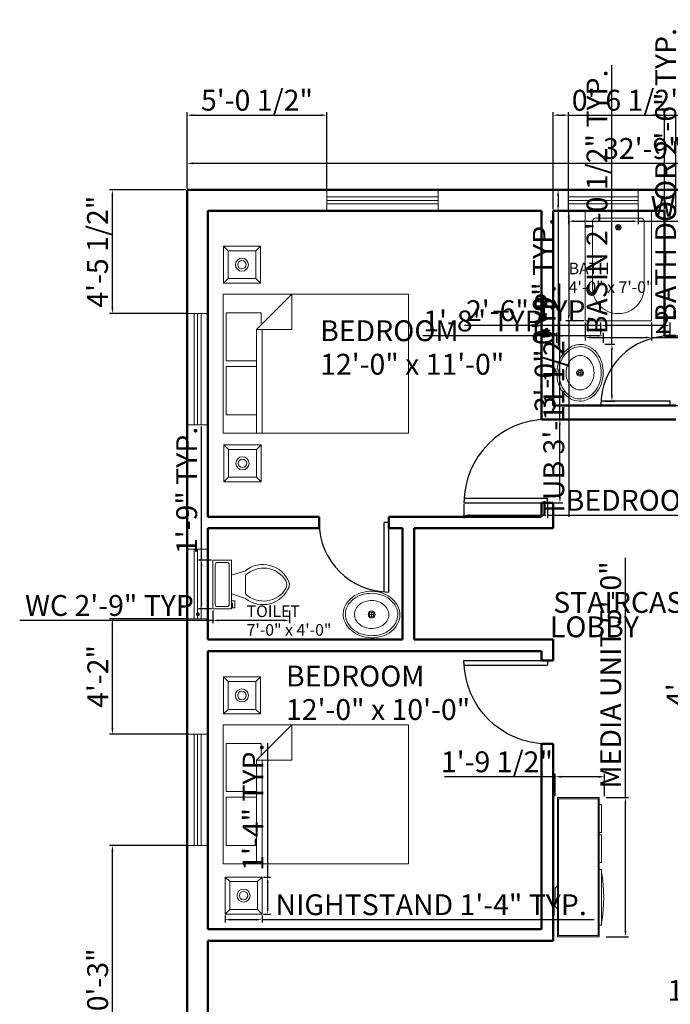
# Model space of a CAD drawing. Units: inches. Extents: x 2866 to 3545, y 873 to 1597.
# Tile 3 of 5: x 2958 to 3239, y 1172 to 1597. Entities that reach past the tile are written whole.
import ezdxf

# ---------------------------------------------------------------- set-up
doc = ezdxf.new("R2010")
doc.units = ezdxf.units.IN
doc.layers.add('A-ANNO-DIMS', color=152, linetype='Continuous', lineweight=18, true_color=0x2776bb)
for name, color, linetype, lineweight in [('A-AREA-IDEN', 7, 'Continuous', 25), ('A-DOOR', 3, 'Continuous', 25), ('A-FLOR-FIXT', 9, 'Continuous', 18), ('A-FURN', 8, 'Continuous', 18), ('A-GLAZ', 4, 'Continuous', 18), ('A-WALL', 7, 'Continuous', 50)]:
    doc.layers.add(name, color=color, linetype=linetype, lineweight=lineweight)
doc.styles.get("Standard").update_dxf_attribs({"font": 'arial.ttf'})
doc.dimstyles.new('ISO-25', dxfattribs={"dimtxt": 9, "dimasz": 2.5, "dimexe": 1.25, "dimexo": 0.625, "dimtad": 1, "dimdec": 0, "dimlunit": 3, "dimtxsty": 'Standard', "dimcen": 4.5, "dimadec": 0, "dimazin": 0, "dimtfac": 1, "dimtdec": 0, "dimtmove": 0, "dimatfit": 3, "dimfxl": 1, "dimarcsym": 0})

# ---------------------------------------------------------------- blocks, each defined once
blk = doc.blocks.new('Toilet - top')
for p, q in [((9.5, -6), (9.5, -2)), ((-8, -8.5), (-8, -8)), ((-7, -8), (-7, -9.5)), ((-4, -8), (-6, -14)), ((4, -8), (6, -14)), ((-10, -8.5), (-8, -8.5)), ((-10, -9.5), (-10, -8.5)), ((-7, -9.5), (-10, -9.5)), ((4, -14), (-4, -14))]:
    blk.add_line(p, q)
blk.add_lwpolyline([(10.5, -8), (10.5, 0), (-10.5, 0), (-10.5, -8)], close=True)
for points in [[(-9.5, -2), (-9.5, -6)], [(8.5, -1), (-8.5, -1)], [(-8.5, -7), (8.5, -7)]]:
    blk.add_lwpolyline(points)
for centre, radius, start, end in [((-8.62, -1.88), 0.884, 81.8699, 188.1301), ((8.62, -1.88), 0.884, 351.8699, 98.1301), ((-8.62, -6.12), 0.884, 171.8699, 278.1301), ((8.62, -6.12), 0.884, 261.8699, 8.1301), ((3.52, -21.58), 12.17, 141.4691, 247.9714), ((4.2, -21.82), 11.33, 136.3677, 238.9468), ((-3.52, -21.58), 12.17, 292.0284, 38.5307), ((-4.2, -21.82), 11.33, 301.053, 43.6321), ((0, -27.88), 4, 245.7318, 294.2682), ((0, -29), 4, 254.8605, 285.1395)]:
    blk.add_arc(centre, radius, start, end)
blk = doc.blocks.new('Entertainment Center')
for p, q in [((-4, 0), (-5, -1)), ((4, 0), (-4, 0)), ((5, -1), (4, 0)), ((-17, -19), (-17, -1)), ((-17, -1), (43, -1)), ((-16.5, -18.5), (-16.5, -1.5)), ((-16.5, -1.5), (42.5, -1.5)), ((42.5, -1.5), (42.5, -18.5)), ((43, -1), (43, -19)), ((43, -19), (-17, -19)), ((42.5, -18.5), (-16.5, -18.5)), ((-12, -20), (-12, -19)), ((12, -20), (-12, -20)), ((12, -19), (12, -20)), ((15, -20), (15, -19)), ((27, -20), (15, -20)), ((27, -19), (27, -20)), ((28, -20), (28, -19)), ((40, -20), (28, -20)), ((40, -19), (40, -20))]:
    blk.add_line(p, q)
blk.add_arc((0, 40), 61, 259.6111, 280.3889)
blk = doc.blocks.new('Bed - Queen')
for p, q in [((0, -80.00003), (0, 0)), ((0, 0), (59.99999, 0)), ((59.99999, 0), (59.99999, -80.00003)), ((7.99999, -1.2), (28.79998, -1.2)), ((7.99999, -14.4), (7.99999, -1.2)), ((28.79998, -1.2), (28.79998, -14.4)), ((31.19999, -1.2), (51.99999, -1.2)), ((31.19999, -14.4), (31.19999, -1.2)), ((51.99999, -1.2), (51.99999, -16.4)), ((0, -14.4), (44.8, -14.4)), ((44.8, -16.8), (0, -16.8)), ((59.99999, -29.6), (44.8, -14.4)), ((44.8, -14.4), (44.8, -29.6)), ((51.99999, -16.4), (46.79936, -16.4)), ((44.8, -29.6), (59.99999, -29.6)), ((59.99999, -80.00003), (0, -80.00003))]:
    blk.add_line(p, q)
blk = doc.blocks.new('Sink - Oval top')
for p, q in [((-1, 0), (1, 0)), ((0, 1), (0, -1))]:
    blk.add_line(p, q)
for points in [[(-12.23, 0.39, 0.117634), (-11.46, -3.36, 0.104469), (-8.88, -6.8, 0.090016), (-5.08, -9.07, 0.08192), (-0.32, -10.02, 0.08192), (4.49, -9.38, 0.090016), (8.42, -7.36, 0.104469), (11.22, -4.09, 0.117634), (12.23, -0.39, 0.117634), (11.46, 3.36, 0.104469), (8.88, 6.8, 0.090016), (5.08, 9.07, 0.08192), (0.32, 10.02, 0.08192), (-4.49, 9.38, 0.090016), (-8.42, 7.36, 0.104469), (-11.22, 4.09, 0.117634)], [(-11.29, 0.16, 0.118622), (-10.52, -3.25, 0.104678), (-8.07, -6.36, 0.089562), (-4.54, -8.37, 0.081185), (-0.13, -9.15, 0.081185), (4.3, -8.49, 0.089562), (7.89, -6.58, 0.104678), (10.42, -3.55, 0.118622), (11.29, -0.16, 0.118622), (10.52, 3.25, 0.104678), (8.07, 6.36, 0.089562), (4.54, 8.37, 0.081185), (0.13, 9.15, 0.081185), (-4.3, 8.49, 0.089562), (-7.89, 6.58, 0.104678), (-10.42, 3.55, 0.118622)], [(-7.42, 0.08, 0.118283), (-6.91, -2.17, 0.104607), (-5.29, -4.21, 0.089718), (-2.97, -5.53, 0.081436), (-0.07, -6.04, 0.081436), (2.84, -5.59, 0.089718), (5.2, -4.33, 0.104607), (6.86, -2.32, 0.118283), (7.42, -0.08, 0.118283), (6.91, 2.17, 0.104607), (5.29, 4.21, 0.089718), (2.97, 5.53, 0.081436), (0.07, 6.04, 0.081436), (-2.84, 5.59, 0.089718), (-5.2, 4.33, 0.104607), (-6.86, 2.32, 0.118283)]]:
    blk.add_lwpolyline(points, format="xyb", close=True)
for radius in [1.5, 1]:
    blk.add_circle((0, 0), radius)
blk = doc.blocks.new('Bath Tub - 26 x 60 in.')
for p, q in [((8, -18), (10, -18)), ((9, -17), (9, -19))]:
    blk.add_line(p, q)
blk.add_lwpolyline([(0, -36), (0, 0), (60, 0), (60, -36)], close=True)
for points in [[(6, -4), (42, -4)], [(4, -30), (4, -6)], [(42, -32), (6, -32)]]:
    blk.add_lwpolyline(points)
for radius in [1.5, 1]:
    blk.add_circle((9, -18), radius)
for centre, radius, start, end in [((5.75, -5.75), 1.77, 81.8699, 188.1301), ((42, -18), 14, 270, 90), ((5.75, -30.25), 1.77, 171.8699, 278.1301)]:
    blk.add_arc(centre, radius, start, end)
blk = doc.blocks.new('*D18')
at = {"layer": 'A-ANNO-DIMS', "color": 0, "lineweight": -2, "transparency": 16777216}
for p, q in [((3265.42, 1329.69), (3246.53, 1329.69)), ((3247.78, 1284.19), (3247.78, 1327.19)), ((3265.42, 1281.69), (3246.53, 1281.69))]:
    blk.add_line(p, q, dxfattribs=at)
at = {"layer": 'A-ANNO-DIMS', "color": 0, "transparency": 16777216}
for points in [[(3247.37, 1327.19), (3248.2, 1327.19), (3247.78, 1329.69)], [(3247.37, 1284.19), (3248.2, 1284.19), (3247.78, 1281.69)]]:
    blk.add_solid(points, dxfattribs=at)
at = {"layer": 'Defpoints', "color": 0, "transparency": 16777216}
for p in [(3247.78, 1329.69), (3266.04, 1329.69), (3266.04, 1281.69)]:
    blk.add_point(p, dxfattribs=at)
at = {"layer": 'A-ANNO-DIMS', "color": 0, "transparency": 16777216, "insert": (3242.66, 1305.69), "char_height": 9, "attachment_point": 5, "rotation": 90}
blk.add_mtext("4'", dxfattribs=at)
blk = doc.blocks.new('*D20')
at = {"layer": 'A-ANNO-DIMS', "color": 0, "lineweight": -2, "transparency": 16777216}
for p, q in [((3030.04, 1524.32), (3030.04, 1536.42)), ((3032.54, 1535.17), (3420.54, 1535.17)), ((3423.04, 1524.32), (3423.04, 1536.42))]:
    blk.add_line(p, q, dxfattribs=at)
at = {"layer": 'A-ANNO-DIMS', "color": 0, "transparency": 16777216}
for points in [[(3032.54, 1535.59), (3032.54, 1534.76), (3030.04, 1535.17)], [(3420.54, 1535.59), (3420.54, 1534.76), (3423.04, 1535.17)]]:
    blk.add_solid(points, dxfattribs=at)
at = {"layer": 'Defpoints', "color": 0, "transparency": 16777216}
for p in [(3423.04, 1535.17), (3030.04, 1523.69), (3423.04, 1523.69)]:
    blk.add_point(p, dxfattribs=at)
at = {"layer": 'A-ANNO-DIMS', "color": 0, "transparency": 16777216, "insert": (3226.54, 1540.4), "char_height": 9, "attachment_point": 5}
blk.add_mtext('32\'-9"', dxfattribs=at)
blk = doc.blocks.new('WIN-48IN')
for p, q in [((0, 0), (0, 48)), ((0, 48), (9, 48)), ((3, 0), (3, 48)), ((4.5, 0), (4.5, 48)), ((6, 0), (6, 48)), ((9, 48), (9, 0)), ((9, 0), (0, 0))]:
    blk.add_line(p, q)
blk = doc.blocks.new('WIN-30IN')
for p, q in [((0, 0), (0, 30)), ((0, 30), (9, 30)), ((3, 0), (3, 30)), ((4.5, 0), (4.5, 30)), ((6, 0), (6, 30)), ((9, 30), (9, 0)), ((9, 0), (0, 0))]:
    blk.add_line(p, q)
blk = doc.blocks.new('BEDSIDE-STAND-16IN')
for p, q in [((0, 16), (2, 14)), ((14, 14), (16, 16)), ((0, 0), (2, 2)), ((16, 0), (14, 2))]:
    blk.add_line(p, q)
for points in [[(0, 16), (16, 16), (16, 0), (0, 0)], [(2, 14), (14, 14), (14, 2), (2, 2)]]:
    blk.add_lwpolyline(points, close=True)
for radius in [2.82, 1.82]:
    blk.add_circle((8, 8), radius)
blk = doc.blocks.new('DOOR-SWING-30IN')
for p, q in [((0, 30), (0, 0)), ((2, 30), (2, 0)), ((0, 0), (2, 0))]:
    blk.add_line(p, q)
blk.add_arc((0, 0), 30, 0, 90)
blk = doc.blocks.new('DOOR-SWING-36IN')
for p, q in [((0, 2), (36, 2)), ((36, 0), (36, 2)), ((0, 0), (36, 0))]:
    blk.add_line(p, q)
blk.add_arc((36, 0), 36, 90, 180)
blk = doc.blocks.new('*D29')
at = {"layer": 'A-ANNO-DIMS', "color": 0, "lineweight": -2, "transparency": 16777216}
for p, q in [((3194.66, 1514.07), (3194.66, 1508.94)), ((3224.66, 1514.07), (3224.66, 1508.94)), ((3197.16, 1510.19), (3222.16, 1510.19)), ((3224.66, 1510.19), (3342.29, 1510.19))]:
    blk.add_line(p, q, dxfattribs=at)
at = {"layer": 'A-ANNO-DIMS', "color": 0, "transparency": 16777216}
for points in [[(3197.16, 1510.61), (3197.16, 1509.78), (3194.66, 1510.19)], [(3222.16, 1510.61), (3222.16, 1509.78), (3224.66, 1510.19)]]:
    blk.add_solid(points, dxfattribs=at)
at = {"layer": 'Defpoints', "color": 0, "transparency": 16777216}
for p in [(3194.66, 1514.69), (3224.66, 1514.69), (3224.66, 1510.19)]:
    blk.add_point(p, dxfattribs=at)
at = {"layer": 'A-ANNO-DIMS', "color": 0, "transparency": 16777216, "insert": (3284.73, 1515.47), "char_height": 9, "attachment_point": 5}
blk.add_mtext('WINDOW 2\'-6" TYP.', dxfattribs=at)
blk = doc.blocks.new('*D30')
at = {"layer": 'A-ANNO-DIMS', "color": 0, "lineweight": -2, "transparency": 16777216}
for p, q in [((3194.03, 1523.69), (3188.91, 1523.69)), ((3190.16, 1521.19), (3190.16, 1517.19)), ((3194.03, 1514.69), (3188.91, 1514.69)), ((3190.16, 1514.69), (3190.16, 1456.08))]:
    blk.add_line(p, q, dxfattribs=at)
at = {"layer": 'A-ANNO-DIMS', "color": 0, "transparency": 16777216}
for points in [[(3189.74, 1521.19), (3190.57, 1521.19), (3190.16, 1523.69)], [(3189.74, 1517.19), (3190.57, 1517.19), (3190.16, 1514.69)]]:
    blk.add_solid(points, dxfattribs=at)
at = {"layer": 'Defpoints', "color": 0, "transparency": 16777216}
for p in [(3194.66, 1523.69), (3190.16, 1514.69), (3194.66, 1514.69)]:
    blk.add_point(p, dxfattribs=at)
at = {"layer": 'A-ANNO-DIMS', "color": 0, "transparency": 16777216, "insert": (3184.94, 1484.14), "char_height": 9, "attachment_point": 5, "rotation": 90}
blk.add_mtext('0\'-9" TYP.', dxfattribs=at)
blk = doc.blocks.new('*D31')
at = {"layer": 'A-ANNO-DIMS', "color": 0, "lineweight": -2, "transparency": 16777216}
for p, q in [((3046.41, 1210.59), (3046.41, 1207.57)), ((3048.91, 1208.82), (3059.91, 1208.82)), ((3062.41, 1210.59), (3062.41, 1207.57)), ((3062.41, 1208.82), (3205.8, 1208.82))]:
    blk.add_line(p, q, dxfattribs=at)
at = {"layer": 'A-ANNO-DIMS', "color": 0, "transparency": 16777216}
for points in [[(3048.91, 1209.23), (3048.91, 1208.4), (3046.41, 1208.82)], [(3059.91, 1209.23), (3059.91, 1208.4), (3062.41, 1208.82)]]:
    blk.add_solid(points, dxfattribs=at)
at = {"layer": 'Defpoints', "color": 0, "transparency": 16777216}
for p in [(3046.41, 1211.22), (3062.41, 1211.22), (3062.41, 1208.82)]:
    blk.add_point(p, dxfattribs=at)
at = {"layer": 'A-ANNO-DIMS', "color": 0, "transparency": 16777216, "insert": (3135.36, 1214.1), "char_height": 9, "attachment_point": 5}
blk.add_mtext('NIGHTSTAND 1\'-4" TYP.', dxfattribs=at)
blk = doc.blocks.new('*D32')
at = {"layer": 'A-ANNO-DIMS', "color": 0, "lineweight": -2, "transparency": 16777216}
for p, q in [((3064.81, 1227.22), (3064.81, 1284.98)), ((3063.04, 1227.22), (3066.06, 1227.22)), ((3064.81, 1213.72), (3064.81, 1224.72)), ((3063.04, 1211.22), (3066.06, 1211.22))]:
    blk.add_line(p, q, dxfattribs=at)
at = {"layer": 'A-ANNO-DIMS', "color": 0, "transparency": 16777216}
for points in [[(3064.39, 1224.72), (3065.23, 1224.72), (3064.81, 1227.22)], [(3064.39, 1213.72), (3065.23, 1213.72), (3064.81, 1211.22)]]:
    blk.add_solid(points, dxfattribs=at)
at = {"layer": 'Defpoints', "color": 0, "transparency": 16777216}
for p in [(3062.41, 1227.22), (3064.81, 1227.22), (3062.41, 1211.22)]:
    blk.add_point(p, dxfattribs=at)
at = {"layer": 'A-ANNO-DIMS', "color": 0, "transparency": 16777216, "insert": (3059.66, 1257.35), "char_height": 9, "attachment_point": 5, "rotation": 90}
blk.add_mtext('1\'-4" TYP.', dxfattribs=at)
blk = doc.blocks.new('*D35')
at = {"layer": 'A-ANNO-DIMS', "color": 0, "lineweight": -2, "transparency": 16777216}
for p, q in [((3243.04, 1460.69), (3243.04, 1597.14)), ((3239.17, 1460.69), (3244.29, 1460.69)), ((3243.04, 1433.19), (3243.04, 1458.19)), ((3239.17, 1430.69), (3244.29, 1430.69))]:
    blk.add_line(p, q, dxfattribs=at)
at = {"layer": 'A-ANNO-DIMS', "color": 0, "transparency": 16777216}
for points in [[(3242.63, 1458.19), (3243.46, 1458.19), (3243.04, 1460.69)], [(3242.63, 1433.19), (3243.46, 1433.19), (3243.04, 1430.69)]]:
    blk.add_solid(points, dxfattribs=at)
at = {"layer": 'Defpoints', "color": 0, "transparency": 16777216}
for p in [(3238.54, 1460.69), (3243.04, 1460.69), (3238.54, 1430.69)]:
    blk.add_point(p, dxfattribs=at)
at = {"layer": 'A-ANNO-DIMS', "color": 0, "transparency": 16777216, "insert": (3237.76, 1530.17), "char_height": 9, "attachment_point": 5, "rotation": 90}
blk.add_mtext('BATH DOOR 2\'-6" TYP.', dxfattribs=at)
blk = doc.blocks.new('*D36')
at = {"layer": 'A-ANNO-DIMS', "color": 0, "lineweight": -2, "transparency": 16777216}
for p, q in [((3208.54, 1461.32), (3208.54, 1466.44)), ((3238.54, 1461.32), (3238.54, 1466.44)), ((3208.54, 1465.19), (3149.78, 1465.19)), ((3236.04, 1465.19), (3211.04, 1465.19))]:
    blk.add_line(p, q, dxfattribs=at)
at = {"layer": 'A-ANNO-DIMS', "color": 0, "transparency": 16777216}
for points in [[(3211.04, 1465.61), (3211.04, 1464.78), (3208.54, 1465.19)], [(3236.04, 1465.61), (3236.04, 1464.78), (3238.54, 1465.19)]]:
    blk.add_solid(points, dxfattribs=at)
at = {"layer": 'Defpoints', "color": 0, "transparency": 16777216}
for p in [(3208.54, 1465.19), (3208.54, 1460.69), (3238.54, 1460.69)]:
    blk.add_point(p, dxfattribs=at)
at = {"layer": 'A-ANNO-DIMS', "color": 0, "transparency": 16777216, "insert": (3177.91, 1470.41), "char_height": 9, "attachment_point": 5}
blk.add_mtext('2\'-6" TYP.', dxfattribs=at)
blk = doc.blocks.new('*D37')
at = {"layer": 'A-ANNO-DIMS', "color": 0, "lineweight": -2, "transparency": 16777216}
for p, q in [((3149.54, 1388.07), (3149.54, 1382.04)), ((3185.54, 1388.07), (3185.54, 1382.04)), ((3152.04, 1383.29), (3183.04, 1383.29)), ((3185.54, 1383.29), (3353.42, 1383.29))]:
    blk.add_line(p, q, dxfattribs=at)
at = {"layer": 'A-ANNO-DIMS', "color": 0, "transparency": 16777216}
for points in [[(3152.04, 1383.71), (3152.04, 1382.88), (3149.54, 1383.29)], [(3183.04, 1383.71), (3183.04, 1382.88), (3185.54, 1383.29)]]:
    blk.add_solid(points, dxfattribs=at)
at = {"layer": 'Defpoints', "color": 0, "transparency": 16777216}
for p in [(3149.54, 1388.69), (3185.54, 1388.69), (3185.54, 1383.29)]:
    blk.add_point(p, dxfattribs=at)
at = {"layer": 'A-ANNO-DIMS', "color": 0, "transparency": 16777216, "insert": (3270.73, 1388.58), "char_height": 9, "attachment_point": 5}
blk.add_mtext('BEDROOM DOOR 3\'-0" TYP.', dxfattribs=at)
blk = doc.blocks.new('*D38')
at = {"layer": 'A-ANNO-DIMS', "color": 0, "lineweight": -2, "transparency": 16777216}
for p, q in [((3190.94, 1424.69), (3190.94, 1483.3)), ((3186.17, 1424.69), (3192.19, 1424.69)), ((3190.94, 1391.19), (3190.94, 1422.19)), ((3186.17, 1388.69), (3192.19, 1388.69))]:
    blk.add_line(p, q, dxfattribs=at)
at = {"layer": 'A-ANNO-DIMS', "color": 0, "transparency": 16777216}
for points in [[(3190.53, 1422.19), (3191.36, 1422.19), (3190.94, 1424.69)], [(3190.53, 1391.19), (3191.36, 1391.19), (3190.94, 1388.69)]]:
    blk.add_solid(points, dxfattribs=at)
at = {"layer": 'Defpoints', "color": 0, "transparency": 16777216}
for p in [(3185.54, 1424.69), (3190.94, 1424.69), (3185.54, 1388.69)]:
    blk.add_point(p, dxfattribs=at)
at = {"layer": 'A-ANNO-DIMS', "color": 0, "transparency": 16777216, "insert": (3185.72, 1455.24), "char_height": 9, "attachment_point": 5, "rotation": 90}
blk.add_mtext('3\'-0" TYP.', dxfattribs=at)
blk = doc.blocks.new('*D39')
at = {"layer": 'A-ANNO-DIMS', "color": 0, "lineweight": -2, "transparency": 16777216}
for p, q in [((3041.19, 1342.27), (3041.19, 1336.69)), ((3074.24, 1342.27), (3074.24, 1336.69)), ((3041.19, 1337.94), (2957.78, 1337.94)), ((3071.74, 1337.94), (3043.69, 1337.94))]:
    blk.add_line(p, q, dxfattribs=at)
at = {"layer": 'A-ANNO-DIMS', "color": 0, "transparency": 16777216}
for points in [[(3043.69, 1338.36), (3043.69, 1337.52), (3041.19, 1337.94)], [(3071.74, 1338.36), (3071.74, 1337.52), (3074.24, 1337.94)]]:
    blk.add_solid(points, dxfattribs=at)
at = {"layer": 'Defpoints', "color": 0, "transparency": 16777216}
for p in [(3041.19, 1342.9), (3074.24, 1342.9), (3041.19, 1337.94)]:
    blk.add_point(p, dxfattribs=at)
at = {"layer": 'A-ANNO-DIMS', "color": 0, "transparency": 16777216, "insert": (2998.23, 1343.22), "char_height": 9, "attachment_point": 5}
blk.add_mtext('WC 2\'-9" TYP.', dxfattribs=at)
blk = doc.blocks.new('*D40')
at = {"layer": 'A-ANNO-DIMS', "color": 0, "lineweight": -2, "transparency": 16777216}
for p, q in [((3036.24, 1363.9), (3036.24, 1421.66)), ((3040.57, 1363.9), (3034.99, 1363.9)), ((3036.24, 1345.4), (3036.24, 1361.4)), ((3040.57, 1342.9), (3034.99, 1342.9))]:
    blk.add_line(p, q, dxfattribs=at)
at = {"layer": 'A-ANNO-DIMS', "color": 0, "transparency": 16777216}
for points in [[(3035.82, 1361.4), (3036.65, 1361.4), (3036.24, 1363.9)], [(3035.82, 1345.4), (3036.65, 1345.4), (3036.24, 1342.9)]]:
    blk.add_solid(points, dxfattribs=at)
at = {"layer": 'Defpoints', "color": 0, "transparency": 16777216}
for p in [(3036.24, 1363.9), (3041.19, 1363.9), (3041.19, 1342.9)]:
    blk.add_point(p, dxfattribs=at)
at = {"layer": 'A-ANNO-DIMS', "color": 0, "transparency": 16777216, "insert": (3031.02, 1394.03), "char_height": 9, "attachment_point": 5, "rotation": 90}
blk.add_mtext('1\'-9" TYP.', dxfattribs=at)
blk = doc.blocks.new('*D41')
at = {"layer": 'A-ANNO-DIMS', "color": 0, "lineweight": -2, "transparency": 16777216}
for p, q in [((3213.39, 1457.07), (3213.39, 1577.48)), ((3210.33, 1457.07), (3214.64, 1457.07)), ((3213.39, 1435.02), (3213.39, 1454.57)), ((3210.33, 1432.52), (3214.64, 1432.52))]:
    blk.add_line(p, q, dxfattribs=at)
at = {"layer": 'A-ANNO-DIMS', "color": 0, "transparency": 16777216}
for points in [[(3212.98, 1454.57), (3213.81, 1454.57), (3213.39, 1457.07)], [(3212.98, 1435.02), (3213.81, 1435.02), (3213.39, 1432.52)]]:
    blk.add_solid(points, dxfattribs=at)
at = {"layer": 'Defpoints', "color": 0, "transparency": 16777216}
for p in [(3209.71, 1457.07), (3213.39, 1457.07), (3209.71, 1432.52)]:
    blk.add_point(p, dxfattribs=at)
at = {"layer": 'A-ANNO-DIMS', "color": 0, "transparency": 16777216, "insert": (3208.11, 1518.53), "char_height": 9, "attachment_point": 5, "rotation": 90}
blk.add_mtext('BASIN 2\'-0 1/2" TYP.', dxfattribs=at)
blk = doc.blocks.new('*D42')
at = {"layer": 'A-ANNO-DIMS', "color": 0, "lineweight": -2, "transparency": 16777216}
for p, q in [((3189.57, 1457.7), (3189.57, 1462.01)), ((3209.71, 1457.7), (3209.71, 1462.01)), ((3189.57, 1460.76), (3131.81, 1460.76)), ((3207.21, 1460.76), (3192.07, 1460.76))]:
    blk.add_line(p, q, dxfattribs=at)
at = {"layer": 'A-ANNO-DIMS', "color": 0, "transparency": 16777216}
for points in [[(3192.07, 1461.17), (3192.07, 1460.34), (3189.57, 1460.76)], [(3207.21, 1461.17), (3207.21, 1460.34), (3209.71, 1460.76)]]:
    blk.add_solid(points, dxfattribs=at)
at = {"layer": 'Defpoints', "color": 0, "transparency": 16777216}
for p in [(3189.57, 1460.76), (3189.57, 1457.07), (3209.71, 1457.07)]:
    blk.add_point(p, dxfattribs=at)
at = {"layer": 'A-ANNO-DIMS', "color": 0, "transparency": 16777216, "insert": (3159.44, 1465.98), "char_height": 9, "attachment_point": 5}
blk.add_mtext('1\'-8" TYP.', dxfattribs=at)
blk = doc.blocks.new('*D51')
at = {"layer": 'A-ANNO-DIMS', "color": 0, "lineweight": -2, "transparency": 16777216}
for p, q in [((3219.23, 1261.48), (3219.23, 1364.88)), ((3210.85, 1261.48), (3220.48, 1261.48)), ((3219.23, 1203.98), (3219.23, 1258.98)), ((3210.85, 1201.48), (3220.48, 1201.48))]:
    blk.add_line(p, q, dxfattribs=at)
at = {"layer": 'A-ANNO-DIMS', "color": 0, "transparency": 16777216}
for points in [[(3218.81, 1258.98), (3219.64, 1258.98), (3219.23, 1261.48)], [(3218.81, 1203.98), (3219.64, 1203.98), (3219.23, 1201.48)]]:
    blk.add_solid(points, dxfattribs=at)
at = {"layer": 'Defpoints', "color": 0, "transparency": 16777216}
for p in [(3210.23, 1261.48), (3219.23, 1261.48), (3210.23, 1201.48)]:
    blk.add_point(p, dxfattribs=at)
at = {"layer": 'A-ANNO-DIMS', "color": 0, "transparency": 16777216, "insert": (3214.01, 1314.43), "char_height": 9, "attachment_point": 5, "rotation": 90}
blk.add_mtext('MEDIA UNIT 5\'-0"', dxfattribs=at)
blk = doc.blocks.new('*D52')
at = {"layer": 'A-ANNO-DIMS', "color": 0, "lineweight": -2, "transparency": 16777216}
for p, q in [((3188.89, 1270.48), (3141.09, 1270.48)), ((3188.89, 1262.11), (3188.89, 1271.73)), ((3207.73, 1270.48), (3191.39, 1270.48)), ((3210.23, 1262.11), (3210.23, 1271.73))]:
    blk.add_line(p, q, dxfattribs=at)
at = {"layer": 'A-ANNO-DIMS', "color": 0, "transparency": 16777216}
for points in [[(3191.39, 1270.9), (3191.39, 1270.06), (3188.89, 1270.48)], [(3207.73, 1270.9), (3207.73, 1270.06), (3210.23, 1270.48)]]:
    blk.add_solid(points, dxfattribs=at)
at = {"layer": 'Defpoints', "color": 0, "transparency": 16777216}
for p in [(3188.89, 1270.48), (3188.89, 1261.48), (3210.23, 1261.48)]:
    blk.add_point(p, dxfattribs=at)
at = {"layer": 'A-ANNO-DIMS', "color": 0, "transparency": 16777216, "insert": (3163.74, 1275.76), "char_height": 9, "attachment_point": 5, "rotation": 360}
blk.add_mtext('1\'-9 1/2"', dxfattribs=at)
blk = doc.blocks.new('*D57')
at = {"layer": 'A-ANNO-DIMS', "color": 0, "lineweight": -2, "transparency": 16777216}
for p, q in [((3201.26, 1514.69), (3193.5, 1514.69)), ((3194.75, 1512.19), (3194.75, 1469.64)), ((3201.26, 1467.14), (3193.5, 1467.14)), ((3194.75, 1467.14), (3194.75, 1382.63))]:
    blk.add_line(p, q, dxfattribs=at)
at = {"layer": 'A-ANNO-DIMS', "color": 0, "transparency": 16777216}
for points in [[(3194.33, 1512.19), (3195.17, 1512.19), (3194.75, 1514.69)], [(3194.33, 1469.64), (3195.17, 1469.64), (3194.75, 1467.14)]]:
    blk.add_solid(points, dxfattribs=at)
at = {"layer": 'Defpoints', "color": 0, "transparency": 16777216}
for p in [(3201.88, 1514.69), (3194.75, 1467.14), (3201.88, 1467.14)]:
    blk.add_point(p, dxfattribs=at)
at = {"layer": 'A-ANNO-DIMS', "color": 0, "transparency": 16777216, "insert": (3189.47, 1423.63), "char_height": 9, "attachment_point": 5, "rotation": 90}
blk.add_mtext('TUB 3\'-11 1/2"', dxfattribs=at)
blk = doc.blocks.new('*D58')
at = {"layer": 'A-ANNO-DIMS', "color": 0, "lineweight": -2, "transparency": 16777216}
for p, q in [((3201.88, 1466.51), (3201.88, 1458.75)), ((3230.42, 1466.51), (3230.42, 1458.75)), ((3204.38, 1460), (3227.92, 1460)), ((3230.42, 1460), (3279.22, 1460))]:
    blk.add_line(p, q, dxfattribs=at)
at = {"layer": 'A-ANNO-DIMS', "color": 0, "transparency": 16777216}
for points in [[(3204.38, 1460.42), (3204.38, 1459.59), (3201.88, 1460)], [(3227.92, 1460.42), (3227.92, 1459.59), (3230.42, 1460)]]:
    blk.add_solid(points, dxfattribs=at)
at = {"layer": 'Defpoints', "color": 0, "transparency": 16777216}
for p in [(3201.88, 1467.14), (3230.42, 1467.14), (3230.42, 1460)]:
    blk.add_point(p, dxfattribs=at)
at = {"layer": 'A-ANNO-DIMS', "color": 0, "transparency": 16777216, "insert": (3256.07, 1465.28), "char_height": 9, "attachment_point": 5}
blk.add_mtext('2\'-4 1/2"', dxfattribs=at)
blk = doc.blocks.new('*D63')
at = {"layer": 'A-ANNO-DIMS', "color": 0, "lineweight": -2, "transparency": 16777216}
for p, q in [((3030.04, 1524.32), (3030.04, 1557.19)), ((3032.54, 1555.94), (3087.84, 1555.94)), ((3090.34, 1524.32), (3090.34, 1557.19))]:
    blk.add_line(p, q, dxfattribs=at)
at = {"layer": 'A-ANNO-DIMS', "color": 0, "transparency": 16777216}
for points in [[(3032.54, 1556.36), (3032.54, 1555.53), (3030.04, 1555.94)], [(3087.84, 1556.36), (3087.84, 1555.53), (3090.34, 1555.94)]]:
    blk.add_solid(points, dxfattribs=at)
at = {"layer": 'Defpoints', "color": 0, "transparency": 16777216}
for p in [(3090.34, 1555.94), (3030.04, 1523.69), (3090.34, 1523.69)]:
    blk.add_point(p, dxfattribs=at)
at = {"layer": 'A-ANNO-DIMS', "color": 0, "transparency": 16777216, "insert": (3060.19, 1561.22), "char_height": 9, "attachment_point": 5}
blk.add_mtext('5\'-0 1/2"', dxfattribs=at)
blk = doc.blocks.new('*D65')
at = {"layer": 'A-ANNO-DIMS', "color": 0, "lineweight": -2, "transparency": 16777216}
for p, q in [((3188.04, 1515.32), (3188.04, 1557.19)), ((3190.54, 1555.94), (3192.16, 1555.94)), ((3194.66, 1515.32), (3194.66, 1557.19)), ((3194.66, 1555.94), (3243.3, 1555.94))]:
    blk.add_line(p, q, dxfattribs=at)
at = {"layer": 'A-ANNO-DIMS', "color": 0, "transparency": 16777216}
for points in [[(3190.54, 1556.36), (3190.54, 1555.53), (3188.04, 1555.94)], [(3192.16, 1556.36), (3192.16, 1555.53), (3194.66, 1555.94)]]:
    blk.add_solid(points, dxfattribs=at)
at = {"layer": 'Defpoints', "color": 0, "transparency": 16777216}
for p in [(3194.66, 1555.94), (3188.04, 1514.69), (3194.66, 1514.69)]:
    blk.add_point(p, dxfattribs=at)
at = {"layer": 'A-ANNO-DIMS', "color": 0, "transparency": 16777216, "insert": (3220.23, 1561.22), "char_height": 9, "attachment_point": 5}
blk.add_mtext('0\'-6 1/2"', dxfattribs=at)
blk = doc.blocks.new('*D67')
at = {"layer": 'A-ANNO-DIMS', "color": 0, "lineweight": -2, "transparency": 16777216}
for p, q in [((3233.54, 1555.94), (3231.04, 1555.94)), ((3236.04, 1515.32), (3236.04, 1557.19)), ((3236.04, 1555.94), (3241.04, 1555.94)), ((3241.04, 1515.32), (3241.04, 1557.19)), ((3243.54, 1555.94), (3271.22, 1555.94))]:
    blk.add_line(p, q, dxfattribs=at)
at = {"layer": 'A-ANNO-DIMS', "color": 0, "transparency": 16777216}
for points in [[(3233.54, 1556.36), (3233.54, 1555.53), (3236.04, 1555.94)], [(3243.54, 1556.36), (3243.54, 1555.53), (3241.04, 1555.94)]]:
    blk.add_solid(points, dxfattribs=at)
at = {"layer": 'Defpoints', "color": 0, "transparency": 16777216}
for p in [(3241.04, 1555.94), (3236.04, 1514.69), (3241.04, 1514.69)]:
    blk.add_point(p, dxfattribs=at)
at = {"layer": 'A-ANNO-DIMS', "color": 0, "transparency": 16777216, "insert": (3258.63, 1561.16), "char_height": 9, "attachment_point": 5}
blk.add_mtext('0\'-5"', dxfattribs=at)
blk = doc.blocks.new('*D69')
at = {"layer": 'A-ANNO-DIMS', "color": 0, "lineweight": -2, "transparency": 16777216}
for p, q in [((3029.42, 1240.84), (2996.54, 1240.84)), ((2997.79, 1120.56), (2997.79, 1238.34)), ((3029.42, 1118.06), (2996.54, 1118.06))]:
    blk.add_line(p, q, dxfattribs=at)
at = {"layer": 'A-ANNO-DIMS', "color": 0, "transparency": 16777216}
for points in [[(2997.38, 1238.34), (2998.21, 1238.34), (2997.79, 1240.84)], [(2997.38, 1120.56), (2998.21, 1120.56), (2997.79, 1118.06)]]:
    blk.add_solid(points, dxfattribs=at)
at = {"layer": 'Defpoints', "color": 0, "transparency": 16777216}
for p in [(2997.79, 1240.84), (3030.04, 1240.84), (3030.04, 1118.06)]:
    blk.add_point(p, dxfattribs=at)
at = {"layer": 'A-ANNO-DIMS', "color": 0, "transparency": 16777216, "insert": (2992.57, 1179.45), "char_height": 9, "attachment_point": 5, "rotation": 90}
blk.add_mtext('10\'-3"', dxfattribs=at)
blk = doc.blocks.new('*D70')
at = {"layer": 'A-ANNO-DIMS', "color": 0, "lineweight": -2, "transparency": 16777216}
for p, q in [((3029.42, 1338.69), (2996.54, 1338.69)), ((2997.79, 1291.34), (2997.79, 1336.19)), ((3029.42, 1288.84), (2996.54, 1288.84))]:
    blk.add_line(p, q, dxfattribs=at)
at = {"layer": 'A-ANNO-DIMS', "color": 0, "transparency": 16777216}
for points in [[(2997.38, 1336.19), (2998.21, 1336.19), (2997.79, 1338.69)], [(2997.38, 1291.34), (2998.21, 1291.34), (2997.79, 1288.84)]]:
    blk.add_solid(points, dxfattribs=at)
at = {"layer": 'Defpoints', "color": 0, "transparency": 16777216}
for p in [(2997.79, 1338.69), (3030.04, 1338.69), (3030.04, 1288.84)]:
    blk.add_point(p, dxfattribs=at)
at = {"layer": 'A-ANNO-DIMS', "color": 0, "transparency": 16777216, "insert": (2992.65, 1313.76), "char_height": 9, "attachment_point": 5, "rotation": 90}
blk.add_mtext('4\'-2"', dxfattribs=at)
blk = doc.blocks.new('*D71')
at = {"layer": 'A-ANNO-DIMS', "color": 0, "lineweight": -2, "transparency": 16777216}
for p, q in [((3029.42, 1523.69), (2996.54, 1523.69)), ((2997.79, 1472.86), (2997.79, 1521.19)), ((3029.42, 1470.36), (2996.54, 1470.36))]:
    blk.add_line(p, q, dxfattribs=at)
at = {"layer": 'A-ANNO-DIMS', "color": 0, "transparency": 16777216}
for points in [[(2997.38, 1521.19), (2998.21, 1521.19), (2997.79, 1523.69)], [(2997.38, 1472.86), (2998.21, 1472.86), (2997.79, 1470.36)]]:
    blk.add_solid(points, dxfattribs=at)
at = {"layer": 'Defpoints', "color": 0, "transparency": 16777216}
for p in [(2997.79, 1523.69), (3030.04, 1523.69), (3030.04, 1470.36)]:
    blk.add_point(p, dxfattribs=at)
at = {"layer": 'A-ANNO-DIMS', "color": 0, "transparency": 16777216, "insert": (2992.51, 1497.02), "char_height": 9, "attachment_point": 5, "rotation": 90}
blk.add_mtext('4\'-5 1/2"', dxfattribs=at)

msp = doc.modelspace()

# ---------------------------------------------------------------- linework, layer by layer
at = {"layer": 'A-WALL'}
for p, q in [((3030.04, 1523.69), (3030.04, 1022.69)), ((3030.04, 1523.69), (3423.04, 1523.69)), ((3039.04, 1514.69), (3039.04, 1382.69)), ((3039.04, 1514.69), (3183.04, 1514.69)), ((3183.04, 1514.69), (3183.04, 1424.69)), ((3188.04, 1514.69), (3188.04, 1430.69)), ((3188.04, 1514.69), (3236.04, 1514.69)), ((3236.04, 1514.69), (3236.04, 1460.69)), ((3236.04, 1460.69), (3241.04, 1460.69)), ((3188.04, 1430.69), (3241.04, 1430.69)), ((3183.04, 1424.69), (3188.04, 1424.69)), ((3183.04, 1424.69), (3241.04, 1424.69)), ((3236.04, 1424.69), (3241.04, 1424.69)), ((3183.04, 1388.69), (3183.04, 1382.69)), ((3183.04, 1388.69), (3188.04, 1388.69)), ((3188.04, 1388.69), (3188.04, 1377.69)), ((3039.04, 1382.69), (3087.04, 1382.69)), ((3087.04, 1382.69), (3087.04, 1377.69)), ((3117.04, 1382.69), (3117.04, 1377.69)), ((3117.04, 1382.69), (3183.04, 1382.69)), ((3039.04, 1377.69), (3087.04, 1377.69)), ((3039.04, 1377.69), (3039.04, 1329.69)), ((3117.04, 1377.69), (3123.04, 1377.69)), ((3123.04, 1377.69), (3123.04, 1329.69)), ((3128.04, 1377.69), (3128.04, 1329.69)), ((3128.04, 1377.69), (3188.04, 1377.69)), ((3039.04, 1329.69), (3123.04, 1329.69)), ((3128.04, 1329.69), (3188.04, 1329.69)), ((3188.04, 1329.69), (3188.04, 1320.69)), ((3039.04, 1324.69), (3183.04, 1324.69)), ((3039.04, 1324.69), (3039.04, 1204.69)), ((3183.04, 1324.69), (3183.04, 1320.69)), ((3183.04, 1320.69), (3188.04, 1320.69)), ((3183.04, 1284.69), (3183.04, 1204.69)), ((3183.04, 1284.69), (3188.04, 1284.69)), ((3188.04, 1284.69), (3188.04, 1199.69)), ((3039.04, 1204.69), (3183.04, 1204.69)), ((3039.04, 1199.69), (3188.04, 1199.69)), ((3039.04, 1199.69), (3039.04, 1031.69))]:
    msp.add_line(p, q, dxfattribs=at)

# ---------------------------------------------------------------- block references
at = {"layer": 'A-DOOR'}
for p, rotation in [((3238.54, 1430.69), 90.00000000000087), ((3117.04, 1380.19), 180)]:
    msp.add_blockref('DOOR-SWING-30IN', p, dxfattribs=dict(at, rotation=rotation))
msp.add_blockref('DOOR-SWING-36IN', (3149.54, 1388.69), dxfattribs=at)
at = {"layer": 'A-DOOR', "extrusion": (0, 0, -1), "zscale": -1, "rotation": 180}
msp.add_blockref('DOOR-SWING-36IN', (-3149.54, 1320.69), dxfattribs=at)
at = {"layer": 'A-FLOR-FIXT', "xscale": 0.792588089790706, "yscale": 0.792588089790706, "zscale": 0.792588089790706, "rotation": 270}
msp.add_blockref('Bath Tub - 26 x 60 in.', (3230.42, 1514.69), dxfattribs=at)
at = {"layer": 'A-FLOR-FIXT', "rotation": 90}
for name, p in [('Sink - Oval top', (3199.64, 1444.8)), ('Toilet - top', (3041.19, 1353.4))]:
    msp.add_blockref(name, p, dxfattribs=at)
at = {"layer": 'A-FLOR-FIXT'}
msp.add_blockref('Sink - Oval top', (3109.67, 1340.49), dxfattribs=at)
at = {"layer": 'A-FURN'}
for p in [(3045.72, 1483.43), (3045.94, 1397.71), (3045.7, 1297.56), (3046.41, 1211.22)]:
    msp.add_blockref('BEDSIDE-STAND-16IN', p, dxfattribs=at)
for name, p, rotation in [('Bed - Queen', (3045.64, 1418.69), 89.99999999999999), ('Bed - Queen', (3045.64, 1232.87), 89.99999999999999), ('Entertainment Center', (3188.89, 1218.48), 89.9999967828676)]:
    msp.add_blockref(name, p, dxfattribs=dict(at, rotation=rotation))
at = {"layer": 'A-GLAZ', "rotation": 270}
for name, p in [('WIN-48IN', (3090.34, 1523.69)), ('WIN-30IN', (3194.66, 1523.69))]:
    msp.add_blockref(name, p, dxfattribs=at)
at = {"layer": 'A-GLAZ'}
for name, p in [('WIN-48IN', (3030.04, 1422.36)), ('WIN-30IN', (3030.04, 1338.69)), ('WIN-48IN', (3030.04, 1240.84))]:
    msp.add_blockref(name, p, dxfattribs=at)

# ---------------------------------------------------------------- texts
at = {"layer": 'A-AREA-IDEN'}
for s, height, p in [('BATH', 5, (3194.74, 1487.28)), ('4\'-0" x 7\'-0"', 5, (3194.74, 1479.24)), ('BEDROOM', 9, (3087.46, 1458.43)), ('12\'-0" x 11\'-0"', 9, (3087.46, 1443.97)), ('STAIRCASE', 9, (3188.07, 1341.21)), ('TOILET', 5, (3055.72, 1339.38)), ('LOBBY', 9, (3186.63, 1330.67)), ('7\'-0" x 4\'-0"', 5, (3055.72, 1331.35)), ('BEDROOM', 9, (3072.72, 1309.43)), ('12\'-0" x 10\'-0"', 9, (3072.72, 1294.98)), ('18\'-10" x 15\'-0"', 9, (3237.41, 1173.8))]:
    msp.add_text(s, height=height, dxfattribs=at).set_placement(p)

# ---------------------------------------------------------------- dimensions: what is measured, and where the dimension line sits
at = {"layer": 'A-ANNO-DIMS'}
for base, p1, p2, angle, text, picture, middle in [((3243.04, 1460.69), (3238.54, 1430.69), (3238.54, 1460.69), 90, 'BATH DOOR <> TYP.', '*D35', (3237.76, 1530.17)), ((3213.3924, 1457.0738), (3209.7098, 1432.5229), (3209.7098, 1457.0738), 90, 'BASIN <> TYP.', '*D41', (3208.114, 1518.5269)), ((3190.16, 1514.69), (3194.66, 1523.69), (3194.66, 1514.69), 270, '<> TYP.', '*D30', (3184.94, 1484.14)), ((3194.7502, 1467.1364), (3201.8835, 1514.6917), (3201.8835, 1467.1364), 270, 'TUB <>', '*D57', (3189.4687, 1423.6342)), ((3208.54, 1465.19), (3238.54, 1460.69), (3208.54, 1460.69), 180, '<> TYP.', '*D36', (3177.91, 1470.41)), ((3190.94, 1424.69), (3185.54, 1388.69), (3185.54, 1424.69), 90, '<> TYP.', '*D38', (3185.72, 1455.24)), ((3189.57, 1460.76), (3209.71, 1457.07), (3189.57, 1457.07), 180, '<> TYP.', '*D42', (3159.44, 1465.98)), ((3036.24, 1363.9), (3041.19, 1342.9), (3041.19, 1363.9), 90, '<> TYP.', '*D40', (3031.02, 1394.03)), ((3041.1933, 1337.9402), (3074.2395, 1342.8972), (3041.1933, 1342.8972), 180, 'WC <> TYP.', '*D39', (2998.2344, 1343.2187)), ((3219.23, 1261.48), (3210.23, 1201.48), (3210.23, 1261.48), 90, 'MEDIA UNIT <>', '*D51', (3214.01, 1314.43)), ((3064.81, 1227.22), (3062.41, 1211.22), (3062.41, 1227.22), 90, '<> TYP.', '*D32', (3059.66, 1257.35))]:
    dim = msp.add_linear_dim(base=base, p1=p1, p2=p2, angle=angle, text=text, dimstyle='ISO-25', override={"dimdec": 1, "dimlfac": 1, "dimrnd": 0, "dimzin": 1, "dimdsep": 46, "dimlunit": 4, "dimfrac": 2}, dxfattribs=at)
    dim.commit()
    dim.dimension.update_dxf_attribs({"geometry": picture, "text_midpoint": middle})
for base, p1, p2, override, picture, middle in [((3090.34, 1555.94), (3030.04, 1523.69), (3090.34, 1523.69), {"dimdec": 1, "dimlfac": 1, "dimrnd": 0, "dimzin": 1, "dimdsep": 46, "dimlunit": 4, "dimfrac": 2}, '*D63', (3060.19, 1561.22)), ((3194.66, 1555.94), (3188.04, 1514.69), (3194.66, 1514.69), {"dimdec": 1, "dimlfac": 1, "dimrnd": 0, "dimzin": 1, "dimdsep": 46, "dimlunit": 4, "dimfrac": 2}, '*D65', (3220.23, 1561.22)), ((3241.04, 1555.94), (3236.04, 1514.69), (3241.04, 1514.69), {"dimdec": 1, "dimlfac": 1, "dimrnd": 0, "dimzin": 1, "dimdsep": 46, "dimlunit": 4, "dimfrac": 2}, '*D67', (3258.63, 1561.16)), ((3423.04, 1535.17), (3030.04, 1523.69), (3423.04, 1523.69), {"dimclrd": 0, "dimclre": 0, "dimclrt": 0}, '*D20', (3226.54, 1540.4)), ((3230.42, 1460), (3201.88, 1467.14), (3230.42, 1467.14), {"dimdec": 1, "dimlfac": 1, "dimrnd": 0, "dimzin": 1, "dimdsep": 46, "dimlunit": 4, "dimfrac": 2}, '*D58', (3256.07, 1465.28))]:
    dim = msp.add_linear_dim(base=base, p1=p1, p2=p2, dimstyle='ISO-25', override=override, dxfattribs=at)
    dim.commit()
    dim.dimension.update_dxf_attribs({"geometry": picture, "text_midpoint": middle})
for base, p1, p2, text, picture, middle in [((3224.66, 1510.19), (3194.66, 1514.69), (3224.66, 1514.69), 'WINDOW <> TYP.', '*D29', (3284.73, 1515.47)), ((3185.54, 1383.29), (3149.54, 1388.69), (3185.54, 1388.69), 'BEDROOM DOOR <> TYP.', '*D37', (3270.73, 1388.58)), ((3062.41, 1208.82), (3046.41, 1211.22), (3062.41, 1211.22), 'NIGHTSTAND <> TYP.', '*D31', (3135.36, 1214.1))]:
    dim = msp.add_linear_dim(base=base, p1=p1, p2=p2, text=text, dimstyle='ISO-25', override={"dimdec": 1, "dimlfac": 1, "dimrnd": 0, "dimzin": 1, "dimdsep": 46, "dimlunit": 4, "dimfrac": 2}, dxfattribs=at)
    dim.commit()
    dim.dimension.update_dxf_attribs({"geometry": picture, "text_midpoint": middle})
for base, p1, p2, angle, override, picture, middle in [((2997.79, 1523.69), (3030.04, 1470.36), (3030.04, 1523.69), 90, {"dimdec": 1, "dimlfac": 1, "dimrnd": 0, "dimzin": 1, "dimdsep": 46, "dimlunit": 4, "dimfrac": 2}, '*D71', (2992.51, 1497.02)), ((2997.7917, 1338.6917), (3030.0417, 1288.8362), (3030.0417, 1338.6917), 90, {"dimdec": 1, "dimlfac": 1, "dimrnd": 0, "dimzin": 1, "dimdsep": 46, "dimlunit": 4, "dimfrac": 2}, '*D70', (2992.6483, 1313.7639)), ((3247.78, 1329.69), (3266.04, 1281.69), (3266.04, 1329.69), 90, {"dimclrd": 0, "dimclre": 0, "dimclrt": 0}, '*D18', (3242.66, 1305.69)), ((3188.89, 1270.48), (3210.23, 1261.48), (3188.89, 1261.48), 180, {"dimdec": 1, "dimlfac": 1, "dimrnd": 0, "dimzin": 1, "dimdsep": 46, "dimlunit": 4, "dimfrac": 2}, '*D52', (3163.74, 1275.76)), ((2997.79, 1240.84), (3030.04, 1118.06), (3030.04, 1240.84), 90, {"dimdec": 1, "dimlfac": 1, "dimrnd": 0, "dimzin": 1, "dimdsep": 46, "dimlunit": 4, "dimfrac": 2}, '*D69', (2992.57, 1179.45))]:
    dim = msp.add_linear_dim(base=base, p1=p1, p2=p2, angle=angle, dimstyle='ISO-25', override=override, dxfattribs=at)
    dim.commit()
    dim.dimension.update_dxf_attribs({"geometry": picture, "text_midpoint": middle})

doc.saveas('drawing.dxf')
